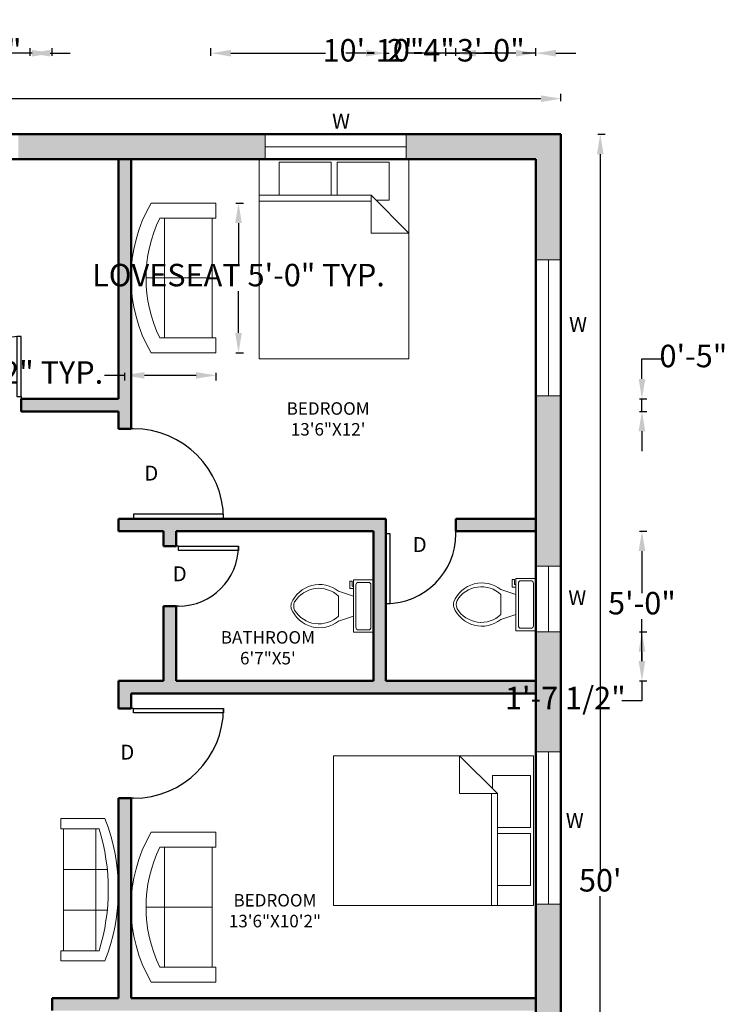
# Model space of a CAD drawing. Units: inches. Extents: x 2568 to 3190, y 746 to 1467.
# Tile 7 of 7: x 2898 to 3181, y 1073 to 1467. Entities that reach past the tile are written whole.
import ezdxf

# ---------------------------------------------------------------- set-up
doc = ezdxf.new("R2010")
doc.units = ezdxf.units.IN
for name, color, linetype, lineweight in [('A-ANNO-DIMS', 2, 'Continuous', 18), ('A-ANNO-TEXT', 7, 'Continuous', 18), ('A-AREA-IDEN', 7, 'Continuous', 25), ('A-DOOR', 3, 'Continuous', 25), ('A-FLOR-FIXT', 9, 'Continuous', 20), ('A-FURN', 8, 'Continuous', 18), ('A-GLAZ', 4, 'Continuous', 20), ('A-WALL', 7, 'Continuous', 50), ('A-WALL-PATT', 252, 'Continuous', 13)]:
    doc.layers.add(name, color=color, linetype=linetype, lineweight=lineweight)
doc.styles.get("Standard").update_dxf_attribs({"font": 'arial.ttf'})
doc.dimstyles.new('ISO-25', dxfattribs={"dimtxt": 9, "dimasz": 8, "dimexe": 2, "dimexo": 1, "dimtad": 0, "dimtih": 1, "dimtoh": 1, "dimdec": 1, "dimlunit": 3, "dimtxsty": 'Standard', "dimcen": 2.5, "dimclrd": 1, "dimclre": 3, "dimclrt": 6, "dimadec": 0, "dimazin": 0, "dimtfac": 1, "dimtdec": 1, "dimtmove": 0, "dimatfit": 3, "dimfxl": 1, "dimfxlon": 1, "dimarcsym": 0})

# ---------------------------------------------------------------- blocks, each defined once
blk = doc.blocks.new('*U6')
for p, q in [((0, 0), (0, 6)), ((28, 0), (28, 6))]:
    blk.add_line(p, q)
blk.add_lwpolyline([(0, 0), (0, -28), (1.75, -28), (1.75, 0)], close=True)
blk.add_arc((0, 0), 28, 270, 0)
blk = doc.blocks.new('*U2')
for p, q in [((-24, 0), (-24, -6)), ((0, 0), (0, -6))]:
    blk.add_line(p, q)
blk.add_lwpolyline([(0, 0), (0, 24), (-1.75, 24), (-1.75, 0)], close=True)
blk.add_arc((0, 0), 24, 90, 180)
blk = doc.blocks.new('*U3')
for p, q in [((0, 0), (0, -6)), ((24, 0), (24, -6))]:
    blk.add_line(p, q)
blk.add_lwpolyline([(0, 0), (0, 24), (1.75, 24), (1.75, 0)], close=True)
blk.add_arc((0, 0), 24, 0, 90)
blk = doc.blocks.new('*U4')
for p, q in [((0, 0), (0, -6)), ((-36, 0), (-36, -6))]:
    blk.add_line(p, q)
blk.add_lwpolyline([(0, 0), (0, 36), (-1.75, 36), (-1.75, 0)], close=True)
blk.add_arc((0, 0), 36, 90, 180)
blk = doc.blocks.new('*U7')
for p, q in [((0, 0), (0, -6)), ((36, 0), (36, -6))]:
    blk.add_line(p, q)
blk.add_lwpolyline([(0, 0), (0, 36), (1.75, 36), (1.75, 0)], close=True)
blk.add_arc((0, 0), 36, 0, 90)
blk = doc.blocks.new('Bed - Queen')
for p, q in [((0, -80.00003), (0, 0)), ((0, 0), (59.99999, 0)), ((59.99999, 0), (59.99999, -80.00003)), ((7.99999, -1.2), (28.79998, -1.2)), ((7.99999, -14.4), (7.99999, -1.2)), ((28.79998, -1.2), (28.79998, -14.4)), ((31.19999, -1.2), (51.99999, -1.2)), ((31.19999, -14.4), (31.19999, -1.2)), ((51.99999, -1.2), (51.99999, -16.4)), ((0, -14.4), (44.8, -14.4)), ((59.99999, -29.6), (44.8, -14.4)), ((44.8, -14.4), (44.8, -29.6)), ((44.8, -16.8), (0, -16.8)), ((51.99999, -16.4), (46.79936, -16.4)), ((44.8, -29.6), (59.99999, -29.6)), ((59.99999, -80.00003), (0, -80.00003))]:
    blk.add_line(p, q)
blk = doc.blocks.new('Toilet - top')
for p, q in [((9.5, -6), (9.5, -2)), ((-10, -8.5), (-8, -8.5)), ((-10, -9.5), (-10, -8.5)), ((-7, -9.5), (-10, -9.5)), ((-8, -8.5), (-8, -8)), ((-7, -8), (-7, -9.5)), ((-4, -8), (-6, -14)), ((4, -8), (6, -14)), ((4, -14), (-4, -14))]:
    blk.add_line(p, q)
blk.add_lwpolyline([(10.5, -8), (10.5, 0), (-10.5, 0), (-10.5, -8)], close=True)
for points in [[(-9.5, -2), (-9.5, -6)], [(8.5, -1), (-8.5, -1)], [(-8.5, -7), (8.5, -7)]]:
    blk.add_lwpolyline(points)
for centre, radius, start, end in [((-8.62, -1.88), 0.884, 81.8699, 188.1301), ((8.62, -1.88), 0.884, 351.8699, 98.1301), ((-8.62, -6.12), 0.884, 171.8699, 278.1301), ((8.62, -6.12), 0.884, 261.8699, 8.1301), ((3.52, -21.58), 12.17, 141.4691, 247.9714), ((4.2, -21.82), 11.33, 136.3677, 238.9468), ((-3.52, -21.58), 12.17, 292.0284, 38.5307), ((-4.2, -21.82), 11.33, 301.053, 43.6321), ((0, -27.88), 4, 245.7318, 294.2682), ((0, -29), 4, 254.8605, 285.1395)]:
    blk.add_arc(centre, radius, start, end)
blk = doc.blocks.new('Sofa - Roundback 7 ft.')
for p, q in [((-36.000027, -34), (-36.000027, -11.4696)), ((-12.00002, -32.4421), (-12.00003, -6.5971)), ((11.99997, -32.4421), (11.99998, -6.5971)), ((35.99998, -34), (35.99998, -11.4696)), ((-35.999844, -13.3819), (35.9998, -13.3819)), ((-36.000027, -32.4421), (35.99998, -32.4421))]:
    blk.add_line(p, q)
for points in [[(-36.000027, -34), (-42.000027, -34), (-42.000027, -8)], [(41.99998, -8), (41.99998, -34), (35.99998, -34)]]:
    blk.add_lwpolyline(points)
for centre, radius, start, end in [((0, -114.25), 114.25, 68.43141, 111.5686), ((-0.00001, -127.1968), 121.1968, 72.72033, 107.2797)]:
    blk.add_arc(centre, radius, start, end)
blk = doc.blocks.new('*D13')
at = {"layer": 'A-ANNO-DIMS', "color": 0, "lineweight": -2, "transparency": 16777216}
for p, q in [((2634.52, 1434.58), (2634.52, 1437.58)), ((2642.52, 1435.58), (2866.08, 1435.58)), ((3106.52, 1435.58), (2882.97, 1435.58)), ((3114.52, 1434.58), (3114.52, 1437.58))]:
    blk.add_line(p, q, dxfattribs=at)
at = {"layer": 'A-ANNO-DIMS', "color": 0, "transparency": 16777216}
for points in [[(2642.52, 1436.91), (2642.52, 1434.24), (2634.52, 1435.58)], [(3106.52, 1436.91), (3106.52, 1434.24), (3114.52, 1435.58)]]:
    blk.add_solid(points, dxfattribs=at)
at = {"layer": 'Defpoints', "color": 0, "transparency": 16777216}
for p in [(2634.52, 1435.58), (2634.52, 1421.35), (3114.52, 1421.35)]:
    blk.add_point(p, dxfattribs=at)
at = {"layer": 'A-ANNO-DIMS', "color": 0, "transparency": 16777216, "insert": (2874.52, 1435.58), "char_height": 9, "attachment_point": 5}
blk.add_mtext("40'", dxfattribs=at)
blk = doc.blocks.new('*D14')
at = {"layer": 'A-ANNO-DIMS', "color": 0, "lineweight": -2, "transparency": 16777216}
for p, q in [((3129.28, 1421.35), (3132.28, 1421.35)), ((3130.28, 1413.35), (3130.28, 1126.57)), ((3130.28, 829.35), (3130.28, 1116.13)), ((3129.28, 821.35), (3132.28, 821.35))]:
    blk.add_line(p, q, dxfattribs=at)
at = {"layer": 'A-ANNO-DIMS', "color": 0, "transparency": 16777216}
for points in [[(3128.95, 1413.35), (3131.61, 1413.35), (3130.28, 1421.35)], [(3128.95, 829.35), (3131.61, 829.35), (3130.28, 821.35)]]:
    blk.add_solid(points, dxfattribs=at)
at = {"layer": 'Defpoints', "color": 0, "transparency": 16777216}
for p in [(3114.52, 1421.35), (3114.52, 821.35), (3130.28, 821.35)]:
    blk.add_point(p, dxfattribs=at)
at = {"layer": 'A-ANNO-DIMS', "color": 0, "transparency": 16777216, "insert": (3130.28, 1121.35), "char_height": 9, "attachment_point": 5}
blk.add_mtext("50'", dxfattribs=at)
blk = doc.blocks.new('Sofa - Roundback Loveseat 5 ft.')
for p, q in [((0, -32.44198), (0, -5.99998)), ((-24, -33.99998), (-24, -11.46958)), ((24.00004, -33.99998), (24.00004, -11.46958)), ((-23.9998, -13.38178), (23.99986, -13.38178)), ((-24, -32.44198), (24.00004, -32.44198))]:
    blk.add_line(p, q)
for points in [[(-24, -33.99998), (-30, -33.99998), (-30, -7.99998)], [(30.00004, -7.99998), (30.00004, -33.99998), (24.00004, -33.99998)]]:
    blk.add_lwpolyline(points)
for centre, radius, start, end in [((0, -60.24998), 60.24998, 60.13715, 119.8628), ((0, -61.38438), 55.38444, 64.32083, 115.6792)]:
    blk.add_arc(centre, radius, start, end)
blk = doc.blocks.new('WIN-BED-UPPER-54.46')
for p, q in [((5, 54.46), (-5, 54.46)), ((0, 54.46), (0, 0)), ((5, 0), (-5, 0))]:
    blk.add_line(p, q)
blk = doc.blocks.new('WIN-BATH-26.28')
for p, q in [((5, 26.28), (-5, 26.28)), ((0, 0), (0, 26.28)), ((5, 0), (-5, 0))]:
    blk.add_line(p, q)
blk = doc.blocks.new('WIN-BED-MIDDLE-61.03')
for p, q in [((5, 61.03), (-5, 61.03)), ((0, 61.03), (0, 0)), ((5, 0), (-5, 0))]:
    blk.add_line(p, q)
blk = doc.blocks.new('*D23')
at = {"layer": 'A-ANNO-DIMS', "color": 3, "lineweight": -2, "transparency": 16777216}
for p, q in [((2984.52, 1393.76), (2987.52, 1393.76)), ((2984.52, 1333.76), (2987.52, 1333.76))]:
    blk.add_line(p, q, dxfattribs=at)
at = {"layer": 'A-ANNO-DIMS', "color": 1, "lineweight": -2, "transparency": 16777216}
for p, q in [((2985.52, 1385.76), (2985.52, 1369.04)), ((2985.52, 1341.76), (2985.52, 1358.48))]:
    blk.add_line(p, q, dxfattribs=at)
at = {"layer": 'A-ANNO-DIMS', "color": 1, "transparency": 16777216}
for points in [[(2984.19, 1385.76), (2986.86, 1385.76), (2985.52, 1393.76)], [(2984.19, 1341.76), (2986.86, 1341.76), (2985.52, 1333.76)]]:
    blk.add_solid(points, dxfattribs=at)
at = {"layer": 'Defpoints', "color": 0, "transparency": 16777216}
for p in [(2976.52, 1393.76), (2976.52, 1333.76), (2985.52, 1333.76)]:
    blk.add_point(p, dxfattribs=at)
at = {"layer": 'A-ANNO-DIMS', "color": 6, "transparency": 16777216, "insert": (2985.52, 1363.76), "char_height": 9, "attachment_point": 5}
blk.add_mtext('LOVESEAT 5\'-0" TYP.', dxfattribs=at)
blk = doc.blocks.new('*D24')
at = {"layer": 'A-ANNO-DIMS', "color": 3, "lineweight": -2, "transparency": 16777216}
for p, q in [((2939.86, 1325.76), (2939.86, 1322.76)), ((2976.52, 1325.76), (2976.52, 1322.76))]:
    blk.add_line(p, q, dxfattribs=at)
at = {"layer": 'A-ANNO-DIMS', "color": 1, "lineweight": -2, "transparency": 16777216}
for p, q in [((2939.86, 1324.76), (2931.86, 1324.76)), ((2968.52, 1324.76), (2947.86, 1324.76))]:
    blk.add_line(p, q, dxfattribs=at)
at = {"layer": 'A-ANNO-DIMS', "color": 1, "transparency": 16777216}
for points in [[(2947.86, 1326.09), (2947.86, 1323.43), (2939.86, 1324.76)], [(2968.52, 1326.09), (2968.52, 1323.43), (2976.52, 1324.76)]]:
    blk.add_solid(points, dxfattribs=at)
at = {"layer": 'Defpoints', "color": 0, "transparency": 16777216}
for p in [(2939.86, 1333.76), (2976.52, 1333.76), (2939.86, 1324.76)]:
    blk.add_point(p, dxfattribs=at)
at = {"layer": 'A-ANNO-DIMS', "color": 6, "transparency": 16777216, "insert": (2893.32, 1324.76), "char_height": 9, "attachment_point": 5}
blk.add_mtext('3\'-0 1/2" TYP.', dxfattribs=at)
blk = doc.blocks.new('*D43')
at = {"layer": 'A-ANNO-DIMS', "color": 1, "lineweight": -2, "transparency": 16777216}
for p, q in [((2934.52, 759.85), (2926.52, 759.85)), ((2942.52, 759.85), (2946.11, 759.85)), ((2996.2, 759.85), (2992.62, 759.85)), ((3004.2, 759.85), (3012.2, 759.85))]:
    blk.add_line(p, q, dxfattribs=at)
at = {"layer": 'A-ANNO-DIMS', "color": 3, "lineweight": -2, "transparency": 16777216}
for p, q in [((2942.52, 760.85), (2942.52, 757.85)), ((2996.2, 760.85), (2996.2, 757.85))]:
    blk.add_line(p, q, dxfattribs=at)
at = {"layer": 'A-ANNO-DIMS', "color": 1, "transparency": 16777216}
for points in [[(2934.52, 761.18), (2934.52, 758.51), (2942.52, 759.85)], [(3004.2, 761.18), (3004.2, 758.51), (2996.2, 759.85)]]:
    blk.add_solid(points, dxfattribs=at)
at = {"layer": 'Defpoints', "color": 0, "transparency": 16777216}
for p in [(2942.52, 1411.35), (2996.2, 1411.35), (2996.2, 759.85)]:
    blk.add_point(p, dxfattribs=at)
at = {"layer": 'A-ANNO-DIMS', "color": 6, "transparency": 16777216, "insert": (2969.36, 759.85), "char_height": 9, "attachment_point": 5}
blk.add_mtext('4\'-5 1/2"', dxfattribs=at)
blk = doc.blocks.new('*D44')
at = {"layer": 'A-ANNO-DIMS', "color": 1, "lineweight": -2, "transparency": 16777216}
for p, q in [((2988.2, 759.85), (2980.2, 759.85)), ((2996.2, 759.85), (3001.17, 759.85)), ((3052.64, 759.85), (3047.67, 759.85)), ((3060.64, 759.85), (3068.64, 759.85))]:
    blk.add_line(p, q, dxfattribs=at)
at = {"layer": 'A-ANNO-DIMS', "color": 3, "lineweight": -2, "transparency": 16777216}
for p, q in [((2996.2, 760.85), (2996.2, 757.85)), ((3052.64, 760.85), (3052.64, 757.85))]:
    blk.add_line(p, q, dxfattribs=at)
at = {"layer": 'A-ANNO-DIMS', "color": 1, "transparency": 16777216}
for points in [[(2988.2, 761.18), (2988.2, 758.51), (2996.2, 759.85)], [(3060.64, 761.18), (3060.64, 758.51), (3052.64, 759.85)]]:
    blk.add_solid(points, dxfattribs=at)
at = {"layer": 'Defpoints', "color": 0, "transparency": 16777216}
for p in [(2996.2, 1411.35), (3052.64, 1411.35), (3052.64, 759.85)]:
    blk.add_point(p, dxfattribs=at)
at = {"layer": 'A-ANNO-DIMS', "color": 6, "transparency": 16777216, "insert": (3024.42, 759.85), "char_height": 9, "attachment_point": 5}
blk.add_mtext('4\'-8 1/2"', dxfattribs=at)
blk = doc.blocks.new('*D50')
at = {"layer": 'A-ANNO-DIMS', "color": 3, "lineweight": -2, "transparency": 16777216}
for p, q in [((2846.86, 1452.8), (2846.86, 1455.8)), ((2902.21, 1452.8), (2902.21, 1455.8))]:
    blk.add_line(p, q, dxfattribs=at)
at = {"layer": 'A-ANNO-DIMS', "color": 1, "lineweight": -2, "transparency": 16777216}
for p, q in [((2838.86, 1453.8), (2830.86, 1453.8)), ((2846.86, 1453.8), (2851.29, 1453.8)), ((2902.21, 1453.8), (2897.79, 1453.8)), ((2910.21, 1453.8), (2918.21, 1453.8))]:
    blk.add_line(p, q, dxfattribs=at)
at = {"layer": 'A-ANNO-DIMS', "color": 1, "transparency": 16777216}
for points in [[(2838.86, 1455.13), (2838.86, 1452.47), (2846.86, 1453.8)], [(2910.21, 1455.13), (2910.21, 1452.47), (2902.21, 1453.8)]]:
    blk.add_solid(points, dxfattribs=at)
at = {"layer": 'Defpoints', "color": 0, "transparency": 16777216}
for p in [(2902.21, 1453.8), (2846.86, 831.35), (2902.21, 831.35)]:
    blk.add_point(p, dxfattribs=at)
at = {"layer": 'A-ANNO-DIMS', "color": 6, "transparency": 16777216, "insert": (2874.54, 1453.8), "char_height": 9, "attachment_point": 5}
blk.add_mtext('4\'-7 1/2"', dxfattribs=at)
blk = doc.blocks.new('*D53')
at = {"layer": 'A-ANNO-DIMS', "color": 1, "lineweight": -2, "transparency": 16777216}
for p, q in [((3146.97, 1323.35), (3146.97, 1331.35)), ((3146.97, 1331.35), (3154.97, 1331.35)), ((3146.97, 1310.35), (3146.97, 1315.35)), ((3146.97, 1302.35), (3146.97, 1294.35))]:
    blk.add_line(p, q, dxfattribs=at)
at = {"layer": 'A-ANNO-DIMS', "color": 3, "lineweight": -2, "transparency": 16777216}
for p, q in [((3145.97, 1315.35), (3148.97, 1315.35)), ((3145.97, 1310.35), (3148.97, 1310.35))]:
    blk.add_line(p, q, dxfattribs=at)
at = {"layer": 'A-ANNO-DIMS', "color": 1, "transparency": 16777216}
for points in [[(3145.64, 1323.35), (3148.31, 1323.35), (3146.97, 1315.35)], [(3145.64, 1302.35), (3148.31, 1302.35), (3146.97, 1310.35)]]:
    blk.add_solid(points, dxfattribs=at)
at = {"layer": 'Defpoints', "color": 0, "transparency": 16777216}
for p in [(2811.52, 1315.35), (3146.97, 1315.35), (2811.52, 1310.35)]:
    blk.add_point(p, dxfattribs=at)
at = {"layer": 'A-ANNO-DIMS', "color": 6, "transparency": 16777216, "insert": (3167.56, 1331.35), "char_height": 9, "attachment_point": 5}
blk.add_mtext('0\'-5"', dxfattribs=at)
blk = doc.blocks.new('*D54')
at = {"layer": 'A-ANNO-DIMS', "color": 3, "lineweight": -2, "transparency": 16777216}
for p, q in [((2850.52, 760.85), (2850.52, 757.85)), ((2898.52, 760.85), (2898.52, 757.85))]:
    blk.add_line(p, q, dxfattribs=at)
at = {"layer": 'A-ANNO-DIMS', "color": 1, "lineweight": -2, "transparency": 16777216}
for p, q in [((2858.52, 759.85), (2861.75, 759.85)), ((2890.52, 759.85), (2887.29, 759.85))]:
    blk.add_line(p, q, dxfattribs=at)
at = {"layer": 'A-ANNO-DIMS', "color": 1, "transparency": 16777216}
for points in [[(2858.52, 761.18), (2858.52, 758.51), (2850.52, 759.85)], [(2890.52, 761.18), (2890.52, 758.51), (2898.52, 759.85)]]:
    blk.add_solid(points, dxfattribs=at)
at = {"layer": 'Defpoints', "color": 0, "transparency": 16777216}
for p in [(2850.52, 1310.35), (2898.52, 1310.35), (2898.52, 759.85)]:
    blk.add_point(p, dxfattribs=at)
at = {"layer": 'A-ANNO-DIMS', "color": 6, "transparency": 16777216, "insert": (2874.52, 759.85), "char_height": 9, "attachment_point": 5}
blk.add_mtext('4\'-0"', dxfattribs=at)
blk = doc.blocks.new('*D55')
at = {"layer": 'A-ANNO-DIMS', "color": 3, "lineweight": -2, "transparency": 16777216}
for p, q in [((2603.07, 1303.35), (2600.07, 1303.35)), ((2603.07, 1267.35), (2600.07, 1267.35))]:
    blk.add_line(p, q, dxfattribs=at)
at = {"layer": 'A-ANNO-DIMS', "color": 1, "lineweight": -2, "transparency": 16777216}
for p, q in [((2602.07, 1295.35), (2602.07, 1290.57)), ((2602.07, 1275.35), (2602.07, 1280.13))]:
    blk.add_line(p, q, dxfattribs=at)
at = {"layer": 'A-ANNO-DIMS', "color": 1, "transparency": 16777216}
for points in [[(2600.74, 1295.35), (2603.41, 1295.35), (2602.07, 1303.35)], [(2600.74, 1275.35), (2603.41, 1275.35), (2602.07, 1267.35)]]:
    blk.add_solid(points, dxfattribs=at)
at = {"layer": 'Defpoints', "color": 0, "transparency": 16777216}
for p in [(2942.52, 1303.35), (2602.07, 1267.35), (2941.77, 1267.35)]:
    blk.add_point(p, dxfattribs=at)
at = {"layer": 'A-ANNO-DIMS', "color": 6, "transparency": 16777216, "insert": (2602.07, 1285.35), "char_height": 9, "attachment_point": 5}
blk.add_mtext('3\'-0"', dxfattribs=at)
blk = doc.blocks.new('*D57')
at = {"layer": 'A-ANNO-DIMS', "color": 3, "lineweight": -2, "transparency": 16777216}
for p, q in [((2974.52, 1452.8), (2974.52, 1455.8)), ((3104.52, 1452.8), (3104.52, 1455.8))]:
    blk.add_line(p, q, dxfattribs=at)
at = {"layer": 'A-ANNO-DIMS', "color": 1, "lineweight": -2, "transparency": 16777216}
for p, q in [((2982.52, 1453.8), (3020.37, 1453.8)), ((3096.52, 1453.8), (3058.68, 1453.8))]:
    blk.add_line(p, q, dxfattribs=at)
at = {"layer": 'A-ANNO-DIMS', "color": 1, "transparency": 16777216}
for points in [[(2982.52, 1455.13), (2982.52, 1452.47), (2974.52, 1453.8)], [(3096.52, 1455.13), (3096.52, 1452.47), (3104.52, 1453.8)]]:
    blk.add_solid(points, dxfattribs=at)
at = {"layer": 'Defpoints', "color": 0, "transparency": 16777216}
for p in [(3104.52, 1453.8), (2974.52, 1070.35), (3104.52, 1070.35)]:
    blk.add_point(p, dxfattribs=at)
at = {"layer": 'A-ANNO-DIMS', "color": 6, "transparency": 16777216, "insert": (3039.52, 1453.8), "char_height": 9, "attachment_point": 5}
blk.add_mtext('10\'-10"', dxfattribs=at)
blk = doc.blocks.new('*D61')
at = {"layer": 'A-ANNO-DIMS', "color": 3, "lineweight": -2, "transparency": 16777216}
for p, q in [((3068.52, 1452.8), (3068.52, 1455.8)), ((3104.52, 1452.8), (3104.52, 1455.8))]:
    blk.add_line(p, q, dxfattribs=at)
at = {"layer": 'A-ANNO-DIMS', "color": 1, "lineweight": -2, "transparency": 16777216}
for p, q in [((3060.52, 1453.8), (3052.52, 1453.8)), ((3068.52, 1453.8), (3073.94, 1453.8)), ((3104.52, 1453.8), (3099.11, 1453.8)), ((3112.52, 1453.8), (3120.52, 1453.8))]:
    blk.add_line(p, q, dxfattribs=at)
at = {"layer": 'A-ANNO-DIMS', "color": 1, "transparency": 16777216}
for points in [[(3060.52, 1455.13), (3060.52, 1452.47), (3068.52, 1453.8)], [(3112.52, 1455.13), (3112.52, 1452.47), (3104.52, 1453.8)]]:
    blk.add_solid(points, dxfattribs=at)
at = {"layer": 'Defpoints', "color": 0, "transparency": 16777216}
for p in [(3104.52, 1453.8), (3068.52, 1034.35), (3104.52, 1034.35)]:
    blk.add_point(p, dxfattribs=at)
at = {"layer": 'A-ANNO-DIMS', "color": 6, "transparency": 16777216, "insert": (3086.52, 1453.8), "char_height": 9, "attachment_point": 5}
blk.add_mtext('3\'-0"', dxfattribs=at)
blk = doc.blocks.new('*D75')
at = {"layer": 'A-ANNO-DIMS', "color": 3, "lineweight": -2, "transparency": 16777216}
for p, q in [((3044.52, 1452.8), (3044.52, 1455.8)), ((3072.52, 1452.8), (3072.52, 1455.8))]:
    blk.add_line(p, q, dxfattribs=at)
at = {"layer": 'A-ANNO-DIMS', "color": 1, "lineweight": -2, "transparency": 16777216}
for p, q in [((3036.52, 1453.8), (3028.52, 1453.8)), ((3044.52, 1453.8), (3045.86, 1453.8)), ((3072.52, 1453.8), (3071.19, 1453.8)), ((3080.52, 1453.8), (3088.52, 1453.8))]:
    blk.add_line(p, q, dxfattribs=at)
at = {"layer": 'A-ANNO-DIMS', "color": 1, "transparency": 16777216}
for points in [[(3036.52, 1455.13), (3036.52, 1452.47), (3044.52, 1453.8)], [(3080.52, 1455.13), (3080.52, 1452.47), (3072.52, 1453.8)]]:
    blk.add_solid(points, dxfattribs=at)
at = {"layer": 'Defpoints', "color": 0, "transparency": 16777216}
for p in [(3072.52, 1453.8), (3072.52, 1267.35), (3044.52, 1263.1)]:
    blk.add_point(p, dxfattribs=at)
at = {"layer": 'A-ANNO-DIMS', "color": 6, "transparency": 16777216, "insert": (3058.52, 1453.8), "char_height": 9, "attachment_point": 5}
blk.add_mtext('2\'-4"', dxfattribs=at)
blk = doc.blocks.new('*D76')
at = {"layer": 'A-ANNO-DIMS', "color": 3, "lineweight": -2, "transparency": 16777216}
for p, q in [((3044.52, 760.85), (3044.52, 757.85)), ((3104.52, 760.85), (3104.52, 757.85))]:
    blk.add_line(p, q, dxfattribs=at)
at = {"layer": 'A-ANNO-DIMS', "color": 1, "lineweight": -2, "transparency": 16777216}
for p, q in [((3052.52, 759.85), (3061.94, 759.85)), ((3096.52, 759.85), (3087.11, 759.85))]:
    blk.add_line(p, q, dxfattribs=at)
at = {"layer": 'A-ANNO-DIMS', "color": 1, "transparency": 16777216}
for points in [[(3052.52, 761.18), (3052.52, 758.51), (3044.52, 759.85)], [(3096.52, 761.18), (3096.52, 758.51), (3104.52, 759.85)]]:
    blk.add_solid(points, dxfattribs=at)
at = {"layer": 'Defpoints', "color": 0, "transparency": 16777216}
for p in [(3044.52, 1202.35), (3104.52, 1202.35), (3104.52, 759.85)]:
    blk.add_point(p, dxfattribs=at)
at = {"layer": 'A-ANNO-DIMS', "color": 6, "transparency": 16777216, "insert": (3074.52, 759.85), "char_height": 9, "attachment_point": 5}
blk.add_mtext('5\'-0"', dxfattribs=at)
blk = doc.blocks.new('*D77')
at = {"layer": 'A-ANNO-DIMS', "color": 3, "lineweight": -2, "transparency": 16777216}
for p, q in [((3145.97, 1262.35), (3148.97, 1262.35)), ((3145.97, 1202.35), (3148.97, 1202.35))]:
    blk.add_line(p, q, dxfattribs=at)
at = {"layer": 'A-ANNO-DIMS', "color": 1, "lineweight": -2, "transparency": 16777216}
for p, q in [((3146.97, 1254.35), (3146.97, 1237.57)), ((3146.97, 1210.35), (3146.97, 1227.13))]:
    blk.add_line(p, q, dxfattribs=at)
at = {"layer": 'A-ANNO-DIMS', "color": 1, "transparency": 16777216}
for points in [[(3145.64, 1254.35), (3148.31, 1254.35), (3146.97, 1262.35)], [(3145.64, 1210.35), (3148.31, 1210.35), (3146.97, 1202.35)]]:
    blk.add_solid(points, dxfattribs=at)
at = {"layer": 'Defpoints', "color": 0, "transparency": 16777216}
for p in [(3104.52, 1262.35), (3104.52, 1202.35), (3146.97, 1202.35)]:
    blk.add_point(p, dxfattribs=at)
at = {"layer": 'A-ANNO-DIMS', "color": 6, "transparency": 16777216, "insert": (3146.97, 1232.35), "char_height": 9, "attachment_point": 5}
blk.add_mtext('5\'-0"', dxfattribs=at)
blk = doc.blocks.new('*D78')
at = {"layer": 'A-ANNO-DIMS', "color": 3, "lineweight": -2, "transparency": 16777216}
for p, q in [((2603.07, 1256.35), (2600.07, 1256.35)), ((2603.07, 1232.35), (2600.07, 1232.35))]:
    blk.add_line(p, q, dxfattribs=at)
at = {"layer": 'A-ANNO-DIMS', "color": 1, "lineweight": -2, "transparency": 16777216}
for p, q in [((2602.07, 1248.35), (2602.07, 1240.35)), ((2602.07, 1232.35), (2602.07, 1224.35)), ((2602.07, 1224.35), (2594.07, 1224.35))]:
    blk.add_line(p, q, dxfattribs=at)
at = {"layer": 'A-ANNO-DIMS', "color": 1, "transparency": 16777216}
for points in [[(2600.74, 1248.35), (2603.41, 1248.35), (2602.07, 1256.35)], [(2600.74, 1240.35), (2603.41, 1240.35), (2602.07, 1232.35)]]:
    blk.add_solid(points, dxfattribs=at)
at = {"layer": 'Defpoints', "color": 0, "transparency": 16777216}
for p in [(2955.52, 1256.35), (2602.07, 1232.35), (2955.52, 1232.35)]:
    blk.add_point(p, dxfattribs=at)
at = {"layer": 'A-ANNO-DIMS', "color": 6, "transparency": 16777216, "insert": (2581.41, 1224.35), "char_height": 9, "attachment_point": 5}
blk.add_mtext('2\'-0"', dxfattribs=at)
blk = doc.blocks.new('*D79')
at = {"layer": 'A-ANNO-DIMS', "color": 3, "lineweight": -2, "transparency": 16777216}
for p, q in [((3145.97, 1222.08), (3148.97, 1222.08)), ((3145.97, 1202.35), (3148.97, 1202.35))]:
    blk.add_line(p, q, dxfattribs=at)
at = {"layer": 'A-ANNO-DIMS', "color": 1, "lineweight": -2, "transparency": 16777216}
for p, q in [((3146.97, 1214.08), (3146.97, 1210.35)), ((3146.97, 1202.35), (3146.97, 1194.35)), ((3146.97, 1194.35), (3138.97, 1194.35))]:
    blk.add_line(p, q, dxfattribs=at)
at = {"layer": 'A-ANNO-DIMS', "color": 1, "transparency": 16777216}
for points in [[(3145.64, 1214.08), (3148.31, 1214.08), (3146.97, 1222.08)], [(3145.64, 1210.35), (3148.31, 1210.35), (3146.97, 1202.35)]]:
    blk.add_solid(points, dxfattribs=at)
at = {"layer": 'Defpoints', "color": 0, "transparency": 16777216}
for p in [(3104.52, 1222.08), (3104.52, 1202.35), (3146.97, 1202.35)]:
    blk.add_point(p, dxfattribs=at)
at = {"layer": 'A-ANNO-DIMS', "color": 6, "transparency": 16777216, "insert": (3116.32, 1194.35), "char_height": 9, "attachment_point": 5}
blk.add_mtext('1\'-7 1/2"', dxfattribs=at)
blk = doc.blocks.new('*D80')
at = {"layer": 'A-ANNO-DIMS', "color": 3, "lineweight": -2, "transparency": 16777216}
for p, q in [((2838.1, 1452.8), (2838.1, 1455.8)), ((2910.92, 1452.8), (2910.92, 1455.8))]:
    blk.add_line(p, q, dxfattribs=at)
at = {"layer": 'A-ANNO-DIMS', "color": 1, "lineweight": -2, "transparency": 16777216}
for p, q in [((2846.1, 1453.8), (2861.9, 1453.8)), ((2902.92, 1453.8), (2887.12, 1453.8))]:
    blk.add_line(p, q, dxfattribs=at)
at = {"layer": 'A-ANNO-DIMS', "color": 1, "transparency": 16777216}
for points in [[(2846.1, 1455.13), (2846.1, 1452.47), (2838.1, 1453.8)], [(2902.92, 1455.13), (2902.92, 1452.47), (2910.92, 1453.8)]]:
    blk.add_solid(points, dxfattribs=at)
at = {"layer": 'Defpoints', "color": 0, "transparency": 16777216}
for p in [(2910.92, 1453.8), (2838.1, 1075.35), (2910.92, 1075.35)]:
    blk.add_point(p, dxfattribs=at)
at = {"layer": 'A-ANNO-DIMS', "color": 6, "transparency": 16777216, "insert": (2874.51, 1453.8), "char_height": 9, "attachment_point": 5}
blk.add_mtext('6\'-1"', dxfattribs=at)

msp = doc.modelspace()

# ---------------------------------------------------------------- hatches: boundary and pattern name
at = {"layer": 'A-WALL-PATT'}
h = msp.add_hatch(color=256, dxfattribs=at)
h.dxf.hatch_style = 1
h.paths.add_polyline_path([(2709.74, 1411.35), (2709.74, 1421.35), (2634.52, 1421.35), (2634.52, 1371.08), (2644.52, 1371.08), (2644.52, 1411.35)])
h.paths.add_polyline_path([(2844.66, 1411.35), (2844.66, 1421.35), (2763.78, 1421.35), (2763.78, 1411.35)])
h.paths.add_polyline_path([(2996.2, 1411.35), (2996.2, 1421.35), (2897.43, 1421.35), (2897.43, 1411.35)])
h.paths.add_polyline_path([(3104.52, 1411.35), (3104.52, 1371.08), (3114.52, 1371.08), (3114.52, 1421.35), (3052.64, 1421.35), (3052.64, 1411.35)])
h.paths.add_polyline_path([(3114.52, 1316.62), (3104.52, 1316.62), (3104.52, 1248.37), (3114.52, 1248.37)])
h.paths.add_polyline_path([(3104.52, 1174.04), (3114.52, 1174.04), (3114.52, 1222.08), (3104.52, 1222.08)])
h.paths.add_polyline_path([(3104.52, 1020.11), (3114.52, 1020.11), (3114.52, 1113), (3104.52, 1113)])
h.paths.add_polyline_path([(3104.52, 920.42), (3114.52, 920.42), (3114.52, 992.96), (3104.52, 992.96)])
h.paths.add_polyline_path([(3114.52, 821.35), (3114.52, 865.93), (3104.52, 865.93), (3104.52, 831.35), (3055.78, 831.35), (3055.78, 821.35)])
h.paths.add_polyline_path([(2902.21, 831.35), (2902.21, 821.35), (2986.63, 821.35), (2986.63, 831.35)])
h.paths.add_polyline_path([(2634.52, 821.35), (2676.76, 821.35), (2676.76, 831.35), (2644.52, 831.35), (2644.52, 865.93), (2634.52, 865.93)])
h.paths.add_polyline_path([(2754.37, 821.35), (2846.86, 821.35), (2846.86, 831.35), (2754.37, 831.35)])
h.paths.add_polyline_path([(2644.52, 920.42), (2644.52, 1002.57), (2634.52, 1002.57), (2634.52, 920.42)])
h.paths.add_polyline_path([(2644.52, 1044.16), (2644.52, 1113), (2634.52, 1113), (2634.52, 1044.16)])
h.paths.add_polyline_path([(2644.52, 1248.37), (2644.52, 1316.62), (2634.52, 1316.62), (2634.52, 1248.37)])
h.paths.add_polyline_path([(2634.52, 1222.08), (2634.52, 1174.04), (2644.52, 1174.04), (2644.52, 1222.08)])
h = msp.add_hatch(color=256, dxfattribs=at)
h.dxf.hatch_style = 1
h.paths.add_polyline_path([(2811.52, 1411.35), (2806.52, 1411.35), (2806.52, 1303.35), (2811.52, 1303.35), (2811.52, 1310.35), (2850.52, 1310.35), (2850.52, 1315.35), (2811.52, 1315.35)])
h.paths.add_polyline_path([(2942.52, 1411.35), (2937.52, 1411.35), (2937.52, 1315.35), (2898.52, 1315.35), (2898.52, 1310.35), (2937.52, 1310.35), (2937.52, 1303.35), (2942.52, 1303.35)])
h.paths.add_polyline_path([(2811.52, 1267.35), (2704.52, 1267.35), (2704.52, 1261.35), (2704.52, 1237.35), (2704.52, 1202.35), (2644.52, 1202.35), (2644.52, 1197.35), (2806.52, 1197.35), (2806.52, 1191.38), (2811.52, 1191.38), (2811.52, 1202.35), (2793.52, 1202.35), (2793.52, 1232.35), (2788.52, 1232.35), (2788.52, 1202.35), (2709.52, 1202.35), (2709.52, 1262.35), (2788.52, 1262.35), (2788.52, 1256.35), (2793.52, 1256.35), (2793.52, 1262.35), (2811.52, 1262.35)])
h.paths.add_polyline_path([(2680.52, 1267.35), (2644.52, 1267.35), (2644.52, 1261.35), (2680.52, 1261.35)])
h.paths.add_polyline_path([(3044.52, 1267.35), (2937.52, 1267.35), (2937.52, 1262.35), (2955.52, 1262.35), (2955.52, 1256.35), (2960.52, 1256.35), (2960.52, 1262.35), (3039.52, 1262.35), (3039.52, 1202.35), (2960.52, 1202.35), (2960.52, 1232.35), (2955.52, 1232.35), (2955.52, 1202.35), (2937.52, 1202.35), (2937.52, 1191.38), (2942.52, 1191.38), (2942.52, 1197.35), (3104.52, 1197.35), (3104.52, 1202.35), (3044.52, 1202.35)])
h.paths.add_polyline_path([(3104.52, 1267.35), (3072.52, 1267.35), (3072.52, 1262.35), (3104.52, 1262.35)])
h.paths.add_polyline_path([(2838.1, 1075.35), (2811.52, 1075.35), (2811.52, 1155.35), (2806.52, 1155.35), (2806.52, 1075.35), (2644.52, 1075.35), (2644.52, 1070.35), (2806.52, 1070.35), (2811.52, 1070.35), (2838.1, 1070.35)])
h.paths.add_polyline_path([(3104.52, 1075.35), (2942.52, 1075.35), (2942.52, 1155.38), (2937.52, 1155.38), (2937.52, 1075.35), (2910.92, 1075.35), (2910.92, 1070.35), (2937.52, 1070.35), (3104.52, 1070.35)])
h.paths.add_polyline_path([(2811.52, 1038.35), (2806.52, 1038.35), (2806.52, 980.35), (2644.52, 980.35), (2644.52, 975.35), (2806.52, 975.35), (2806.52, 969.37), (2811.52, 969.37), (2811.52, 975.35)])
h.paths.add_polyline_path([(3104.52, 980.35), (2937.52, 980.35), (2937.52, 969.35), (2942.52, 969.35), (2942.52, 975.35), (3104.52, 975.35)])
h.paths.add_polyline_path([(3104.52, 1034.35), (3039.52, 1034.35), (3039.52, 1004.35), (3044.52, 1004.35), (3044.52, 1029.35), (3104.52, 1029.35)])
h.paths.add_polyline_path([(2942.52, 933.35), (2937.52, 933.35), (2937.52, 831.35), (2942.52, 831.35)])
h.paths.add_polyline_path([(2811.52, 933.37), (2806.52, 933.37), (2806.52, 831.35), (2811.52, 831.35)])

# ---------------------------------------------------------------- linework, layer by layer
at = {"layer": 'A-GLAZ'}
for p, q in [((2996.2, 1411.35), (2996.2, 1421.35)), ((3052.64, 1421.35), (3052.64, 1411.35)), ((2996.2, 1416.35), (3052.64, 1416.35))]:
    msp.add_line(p, q, dxfattribs=at)
at = {"layer": 'A-WALL'}
for p, q in [((3114.52, 1421.35), (2634.52, 1421.35)), ((3114.52, 821.35), (3114.52, 1421.35)), ((3104.52, 1411.35), (2644.52, 1411.35)), ((2937.52, 1411.35), (2937.52, 1315.35)), ((2942.52, 1411.35), (2942.52, 1303.35)), ((3104.52, 831.35), (3104.52, 1411.35)), ((2898.52, 1315.35), (2898.52, 1310.35)), ((2898.52, 1315.35), (2937.52, 1315.35)), ((2898.52, 1310.35), (2937.52, 1310.35)), ((2937.52, 1310.35), (2937.52, 1303.35)), ((2937.52, 1303.35), (2942.52, 1303.35)), ((2937.52, 1267.35), (2937.52, 1262.35)), ((3044.52, 1267.35), (2937.52, 1267.35)), ((3044.52, 1202.35), (3044.52, 1267.35)), ((3104.52, 1267.35), (3072.52, 1267.35)), ((3072.52, 1262.35), (3072.52, 1267.35)), ((2937.52, 1262.35), (2955.52, 1262.35)), ((2955.52, 1256.35), (2955.52, 1262.35)), ((2960.52, 1256.35), (2960.52, 1262.35)), ((2960.52, 1262.35), (3039.52, 1262.35)), ((3039.52, 1202.35), (3039.52, 1262.35)), ((3104.52, 1262.35), (3072.52, 1262.35)), ((2960.52, 1256.35), (2955.52, 1256.35)), ((2955.52, 1202.35), (2955.52, 1232.35)), ((2960.52, 1232.35), (2955.52, 1232.35)), ((2960.52, 1202.35), (2960.52, 1232.35)), ((2937.52, 1202.35), (2937.52, 1191.38)), ((2955.52, 1202.35), (2937.52, 1202.35)), ((3039.52, 1202.35), (2960.52, 1202.35)), ((3104.52, 1202.35), (3044.52, 1202.35)), ((3104.52, 1197.35), (2942.52, 1197.35)), ((2942.52, 1197.35), (2942.52, 1191.38)), ((2942.52, 1191.38), (2937.52, 1191.38)), ((2942.52, 1155.38), (2937.52, 1155.38)), ((2937.52, 1155.38), (2937.52, 1075.35)), ((2942.52, 1155.38), (2942.52, 1075.35)), ((2937.52, 1075.35), (2910.92, 1075.35)), ((2910.92, 1075.35), (2910.92, 1070.35)), ((3104.52, 1075.35), (2942.52, 1075.35))]:
    msp.add_line(p, q, dxfattribs=at)

# ---------------------------------------------------------------- block references
at = {"layer": 'A-DOOR'}
for name, p in [('*U2', (2898.52, 1316.35)), ('*U6', (3044.52, 1261.35))]:
    msp.add_blockref(name, p, dxfattribs=at)
at = {"layer": 'A-DOOR', "rotation": 270}
for name, p in [('*U4', (2943.52, 1267.35)), ('*U3', (2961.52, 1256.35)), ('*U7', (2943.52, 1191.38))]:
    msp.add_blockref(name, p, dxfattribs=at)
at = {"layer": 'A-FLOR-FIXT', "rotation": 270}
for p in [(3039.52, 1232.35), (3104.52, 1232.96)]:
    msp.add_blockref('Toilet - top', p, dxfattribs=at)
at = {"layer": 'A-FURN'}
msp.add_blockref('Bed - Queen', (2993.75, 1411.35), dxfattribs=at)
at = {"layer": 'A-FURN', "xscale": -1}
for name, p, rotation in [('Sofa - Roundback Loveseat 5 ft.', (2942.52, 1363.76), 90), ('Bed - Queen', (3103.52, 1112.43), 270), ('Sofa - Roundback Loveseat 5 ft.', (2942.52, 1111.75), 90)]:
    msp.add_blockref(name, p, dxfattribs=dict(at, rotation=rotation))
at = {"layer": 'A-FURN', "xscale": -0.6782133153273913, "yscale": 0.6782133153273913, "zscale": 0.6782133153273913, "rotation": 270}
msp.add_blockref('Sofa - Roundback 7 ft.', (2937.5, 1118.73), dxfattribs=at)
at = {"layer": 'A-GLAZ'}
for name, p in [('WIN-BED-UPPER-54.46', (3109.52, 1316.62)), ('WIN-BATH-26.28', (3109.52, 1222.08)), ('WIN-BED-MIDDLE-61.03', (3109.52, 1113))]:
    msp.add_blockref(name, p, dxfattribs=at)

# ---------------------------------------------------------------- texts
at = {"layer": 'A-ANNO-TEXT', "char_height": 6, "attachment_point": 1}
for s, insert in [('W', (3022.97, 1429.62)), ('W', (3117.82, 1348.18)), ('D', (2947.8, 1288.6)), ('D', (3055.22, 1259.98)), ('D', (2959.19, 1248.28)), ('W', (3117.49, 1238.72)), ('D', (2938.21, 1176.85)), ('W', (3116.5, 1149.51))]:
    msp.add_mtext_dynamic_manual_height_columns(s, width=7.7602, gutter_width=12.5, heights=[0], dxfattribs=dict(at, insert=insert))
at = {"layer": 'A-AREA-IDEN', "char_height": 5, "attachment_point": 1}
for s, insert in [('\\pxqc;BEDROOM\\P13\'6"X12\'', (2986.46, 1313.99)), ('\\pxqc;BATHROOM\\P6\'7"X5\'', (2962.35, 1222.32)), ('\\pxqc;BEDROOM\\P13\'6"X10\'2"', (2965.18, 1117.02))]:
    msp.add_mtext_dynamic_manual_height_columns(s, width=69.8646, gutter_width=12.5, heights=[0], dxfattribs=dict(at, insert=insert))

# ---------------------------------------------------------------- dimensions: what is measured, and where the dimension line sits
at = {"layer": 'A-ANNO-DIMS'}
for base, p1, p2, override, picture, middle in [((2902.2147, 1453.7989), (2846.8636, 831.3489), (2902.2147, 831.3489), {"dimdec": 1, "dimlfac": 1, "dimrnd": 0, "dimzin": 1, "dimdsep": 46, "dimlunit": 4, "dimfrac": 2}, '*D50', (2874.5391, 1453.7989)), ((2910.92, 1453.8), (2838.1, 1075.35), (2910.92, 1075.35), {"dimdec": 1, "dimlfac": 1, "dimrnd": 0, "dimzin": 1, "dimdsep": 46, "dimlunit": 4, "dimfrac": 2}, '*D80', (2874.51, 1453.8)), ((3104.52, 1453.8), (2974.52, 1070.35), (3104.52, 1070.35), {"dimdec": 1, "dimlfac": 1, "dimrnd": 0, "dimzin": 1, "dimdsep": 46, "dimlunit": 4, "dimfrac": 2}, '*D57', (3039.52, 1453.8)), ((3072.52, 1453.8), (3044.52, 1263.1), (3072.52, 1267.35), {"dimdec": 1, "dimlfac": 1, "dimrnd": 0, "dimzin": 1, "dimdsep": 46, "dimlunit": 4, "dimfrac": 2}, '*D75', (3058.52, 1453.8)), ((3104.52, 1453.8), (3068.52, 1034.35), (3104.52, 1034.35), {"dimdec": 1, "dimlfac": 1, "dimrnd": 0, "dimzin": 1, "dimdsep": 46, "dimlunit": 4, "dimfrac": 2}, '*D61', (3086.52, 1453.8)), ((2634.52, 1435.58), (3114.52, 1421.35), (2634.52, 1421.35), {"dimclrd": 0, "dimclre": 0, "dimclrt": 0}, '*D13', (2874.52, 1435.58)), ((2996.2, 759.85), (2942.52, 1411.35), (2996.2, 1411.35), {"dimdec": 1, "dimlfac": 1, "dimrnd": 0, "dimzin": 1, "dimdsep": 46, "dimlunit": 4, "dimfrac": 2}, '*D43', (2969.36, 759.85)), ((3052.64, 759.85), (2996.2, 1411.35), (3052.64, 1411.35), {"dimdec": 1, "dimlfac": 1, "dimrnd": 0, "dimzin": 1, "dimdsep": 46, "dimlunit": 4, "dimfrac": 2}, '*D44', (3024.42, 759.85)), ((2898.52, 759.85), (2850.52, 1310.35), (2898.52, 1310.35), {"dimdec": 1, "dimlfac": 1, "dimrnd": 0, "dimzin": 1, "dimdsep": 46, "dimlunit": 4, "dimfrac": 2}, '*D54', (2874.52, 759.85)), ((3104.52, 759.85), (3044.52, 1202.35), (3104.52, 1202.35), {"dimdec": 1, "dimlfac": 1, "dimrnd": 0, "dimzin": 1, "dimdsep": 46, "dimlunit": 4, "dimfrac": 2}, '*D76', (3074.52, 759.85))]:
    dim = msp.add_linear_dim(base=base, p1=p1, p2=p2, dimstyle='ISO-25', override=override, dxfattribs=at)
    dim.commit()
    dim.dimension.update_dxf_attribs({"geometry": picture, "text_midpoint": middle})
for base, p1, p2, override, picture, middle in [((3130.28, 821.35), (3114.52, 1421.35), (3114.52, 821.35), {"dimclrd": 0, "dimclre": 0, "dimclrt": 0}, '*D14', (3130.28, 1121.35)), ((3146.97, 1315.35), (2811.52, 1310.35), (2811.52, 1315.35), {"dimdec": 1, "dimlfac": 1, "dimrnd": 0, "dimzin": 1, "dimdsep": 46, "dimlunit": 4, "dimfrac": 2}, '*D53', (3167.56, 1331.35)), ((2602.07, 1267.35), (2942.52, 1303.35), (2941.77, 1267.35), {"dimdec": 1, "dimlfac": 1, "dimrnd": 0, "dimzin": 1, "dimdsep": 46, "dimlunit": 4, "dimfrac": 2}, '*D55', (2602.07, 1285.35)), ((3146.97, 1202.35), (3104.52, 1262.35), (3104.52, 1202.35), {"dimdec": 1, "dimlfac": 1, "dimrnd": 0, "dimzin": 1, "dimdsep": 46, "dimlunit": 4, "dimfrac": 2}, '*D77', (3146.97, 1232.35)), ((2602.07, 1232.35), (2955.52, 1256.35), (2955.52, 1232.35), {"dimdec": 1, "dimlfac": 1, "dimrnd": 0, "dimzin": 1, "dimdsep": 46, "dimlunit": 4, "dimfrac": 2}, '*D78', (2581.41, 1224.35)), ((3146.97, 1202.35), (3104.52, 1222.08), (3104.52, 1202.35), {"dimdec": 1, "dimlfac": 1, "dimrnd": 0, "dimzin": 1, "dimdsep": 46, "dimlunit": 4, "dimfrac": 2}, '*D79', (3116.32, 1194.35))]:
    dim = msp.add_linear_dim(base=base, p1=p1, p2=p2, angle=90, dimstyle='ISO-25', override=override, dxfattribs=at)
    dim.commit()
    dim.dimension.update_dxf_attribs({"geometry": picture, "text_midpoint": middle})
for base, p1, p2, angle, text, picture, middle in [((2985.52, 1333.76), (2976.52, 1393.76), (2976.52, 1333.76), 270, 'LOVESEAT <> TYP.', '*D23', (2985.52, 1363.76)), ((2939.86, 1324.76), (2976.52, 1333.76), (2939.86, 1333.76), 180, '<> TYP.', '*D24', (2893.32, 1324.76))]:
    dim = msp.add_linear_dim(base=base, p1=p1, p2=p2, angle=angle, text=text, dimstyle='ISO-25', override={"dimdec": 1, "dimlfac": 1, "dimrnd": 0, "dimzin": 1, "dimdsep": 46, "dimlunit": 4, "dimfrac": 2}, dxfattribs=at)
    dim.commit()
    dim.dimension.update_dxf_attribs({"geometry": picture, "text_midpoint": middle})

doc.saveas('drawing.dxf')
